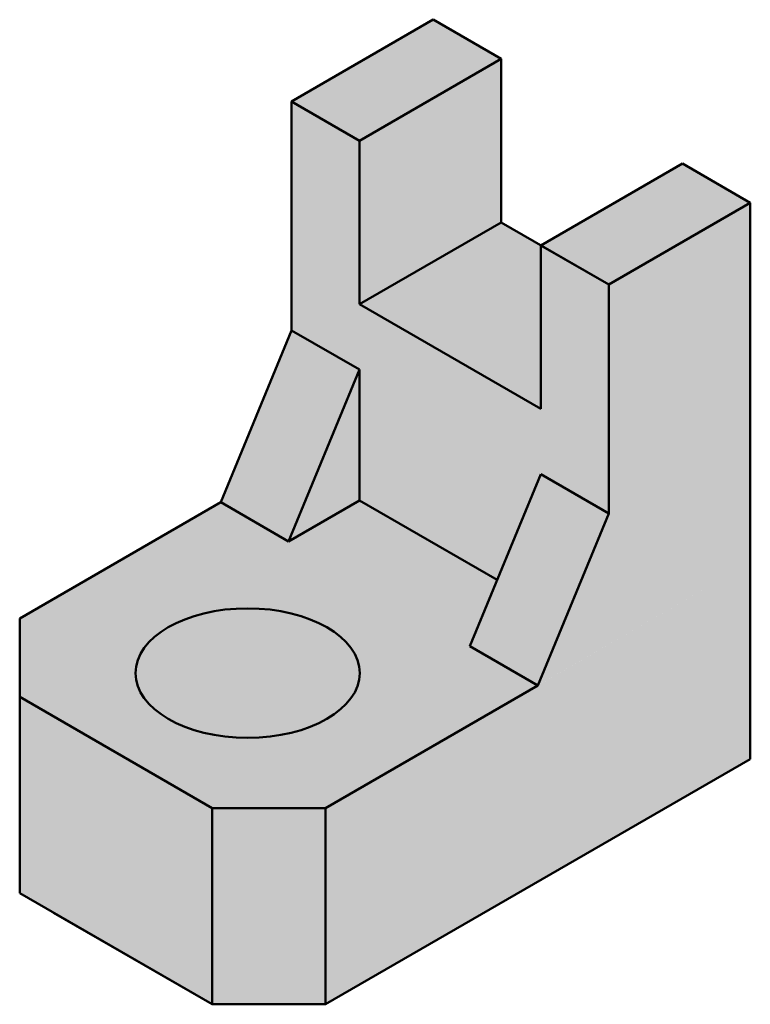
# Model space of a CAD drawing. Units: millimetres. Extents: x 2 to 114, y 2 to 152.
import ezdxf

# ---------------------------------------------------------------- set-up
doc = ezdxf.new("R2010")
doc.units = ezdxf.units.MM
doc.header["$MEASUREMENT"] = 0
doc.layers.add('M-HATC', color=8, linetype='Continuous', lineweight=18)
doc.layers.add('M-OUTL', color=18, linetype='Continuous', lineweight=50)

msp = doc.modelspace()

# ---------------------------------------------------------------- hatches: boundary and pattern name
at = {"layer": 'M-HATC'}
h = msp.add_hatch(color=256, dxfattribs=at)
h.dxf.hatch_style = 1
h.set_gradient(color1=(19, 103, 52), color2=(215, 235, 210), tint=1, name='CYLINDER')
h.paths.add_polyline_path([(81.73, 50.42), (71.34, 56.42), (75.51, 66.54), (54.47, 78.69), (43.62, 72.42), (33.23, 78.42), (2.49, 60.67), (2.49, 48.67), (31.93, 31.67), (49.25, 31.67)])
edge = h.paths.add_edge_path(flags=16)
edge.add_ellipse((37.34, 52.3), major_axis=(-17.15, 0), ratio=0.57735, start_angle=0, end_angle=360)
h.paths.add_polyline_path([(49.25, 31.67), (31.93, 31.67), (31.93, 1.67), (49.25, 1.67)])
h.paths.add_polyline_path([(31.93, 31.67), (2.49, 48.67), (2.49, 18.67), (31.93, 1.67)])
h.paths.add_polyline_path([(114.2, 39.17), (114.21, 69.18), (49.25, 31.67), (49.25, 1.67)])
h.paths.add_polyline_path([(92.58, 76.69), (82.18, 82.69), (71.34, 56.42), (81.73, 50.42)])
h.paths.add_polyline_path([(114.23, 124.19), (92.58, 111.69), (92.58, 86.69), (92.58, 76.69), (81.73, 50.42), (114.21, 69.18)])
h.paths.add_polyline_path([(82.18, 82.69), (92.58, 76.69), (92.58, 86.69), (92.58, 111.69), (82.18, 117.69), (82.18, 92.69), (54.47, 108.69), (54.47, 133.69), (44.08, 139.69), (44.08, 114.69), (44.08, 104.69), (54.47, 98.69), (54.47, 78.69), (75.51, 66.54)])
h.paths.add_polyline_path([(54.47, 98.69), (44.08, 104.69), (33.23, 78.42), (43.62, 72.42)])
h.paths.add_polyline_path([(54.47, 78.69), (54.47, 98.69), (43.62, 72.42)], flags=17)
h.paths.add_polyline_path([(82.18, 117.69), (76.12, 121.19), (54.47, 108.69), (82.18, 92.69)], flags=17)
h.paths.add_polyline_path([(76.12, 146.19), (54.47, 133.69), (54.47, 108.69), (76.12, 121.19)])
h.paths.add_polyline_path([(76.12, 146.19), (65.73, 152.19), (44.08, 139.69), (54.47, 133.69)])
h.paths.add_polyline_path([(114.23, 124.19), (103.84, 130.19), (82.18, 117.69), (92.58, 111.69)])
h = msp.add_hatch(color=256, dxfattribs=at)
h.dxf.hatch_style = 1
h.set_gradient(color1=(19, 103, 52), color2=(215, 235, 210), tint=1)
edge = h.paths.add_edge_path()
edge.add_ellipse((37.34, 52.3), major_axis=(-17.15, 0), ratio=0.57735, start_angle=0, end_angle=360)

# ---------------------------------------------------------------- linework, layer by layer
at = {"layer": 'M-OUTL'}
for p, q in [((44.08, 139.69), (65.73, 152.19)), ((65.73, 152.19), (76.12, 146.19)), ((76.12, 146.19), (54.47, 133.69)), ((76.12, 146.19), (76.12, 121.19)), ((54.47, 133.69), (44.08, 139.69)), ((44.08, 139.69), (44.08, 114.69)), ((54.47, 133.69), (54.47, 108.69)), ((82.18, 117.69), (103.84, 130.19)), ((103.84, 130.19), (114.23, 124.19)), ((114.23, 124.19), (92.58, 111.69)), ((114.23, 124.19), (114.2, 39.17)), ((54.47, 108.69), (76.12, 121.19)), ((76.12, 121.19), (92.58, 111.69)), ((92.58, 111.69), (82.18, 117.69)), ((82.18, 117.69), (82.18, 92.69)), ((44.08, 114.69), (44.08, 104.69)), ((92.58, 111.69), (92.58, 86.69)), ((82.18, 92.69), (54.47, 108.69)), ((44.08, 104.69), (33.23, 78.42)), ((54.47, 98.69), (44.08, 104.69)), ((54.47, 98.69), (43.62, 72.42)), ((54.47, 98.69), (54.47, 78.69)), ((92.58, 86.69), (92.58, 76.69)), ((82.18, 82.69), (71.34, 56.42)), ((92.58, 76.69), (82.18, 82.69)), ((33.23, 78.42), (2.49, 60.67)), ((43.62, 72.42), (33.23, 78.42)), ((43.62, 72.42), (54.47, 78.69)), ((54.47, 78.69), (75.51, 66.54)), ((92.58, 76.69), (81.73, 50.42)), ((2.49, 48.67), (2.49, 60.67)), ((81.73, 50.42), (71.34, 56.42)), ((49.25, 31.67), (81.73, 50.42)), ((31.93, 31.67), (2.49, 48.67)), ((2.49, 48.67), (2.49, 18.67)), ((49.25, 1.67), (114.2, 39.17)), ((31.93, 1.67), (31.93, 31.67)), ((49.25, 31.67), (31.93, 31.67)), ((49.25, 1.67), (49.25, 31.67)), ((31.93, 1.67), (2.49, 18.67)), ((31.93, 1.67), (7.68, 15.67)), ((49.25, 1.67), (31.93, 1.67))]:
    msp.add_line(p, q, dxfattribs=at)
msp.add_ellipse((37.34, 52.3), major_axis=(-17.15, 0), ratio=0.57735, dxfattribs=at)

doc.saveas('drawing.dxf')
